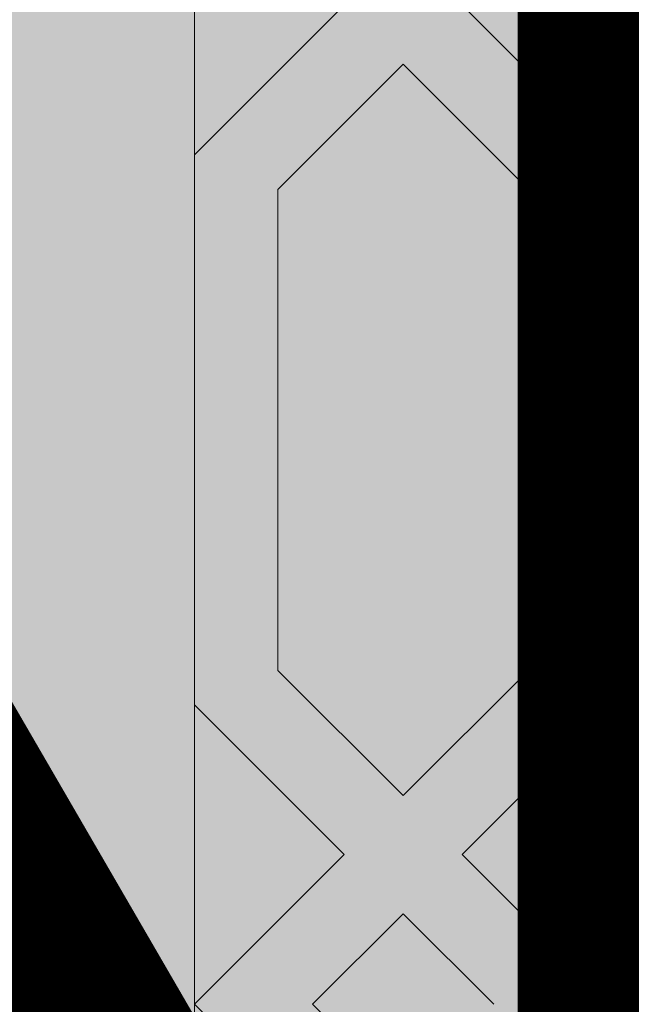
# Model space of a CAD drawing. Units: inches. Extents: x 844 to 2234, y 346 to 1084.
# Tile 83 of 93: x 2008.425 to 2010.294, y 701.365 to 704.373. Entities that reach past the tile are written whole.
import ezdxf

# ---------------------------------------------------------------- set-up
doc = ezdxf.new("R2010")
doc.units = ezdxf.units.IN
doc.header["$MEASUREMENT"] = 0
for name, color, linetype, lineweight in [('A-ANNO-DIMS', 2, 'Continuous', 18), ('furniture', 8, 'Continuous', 18), ('RA-AP-01$0$INT', 35, 'Continuous', 5)]:
    doc.layers.add(name, color=color, linetype=linetype, lineweight=lineweight)
doc.layers.add('RA-AP-01$0$FURN', color=3, linetype='Continuous')
doc.styles.get("Standard").update_dxf_attribs({"font": 'arial.ttf'})
doc.dimstyles.get("Standard").update_dxf_attribs({"dimtxt": 6, "dimasz": 3, "dimexe": 0.18, "dimexo": 0.0625, "dimgap": 0.09, "dimtad": 0, "dimtih": 1, "dimtoh": 1, "dimdec": 1, "dimzin": 0, "dimdsep": 46, "dimlunit": 3, "dimtxsty": 'Standard', "dimblk": 'ARCHTICK', "dimcen": 0.09, "dimadec": 0, "dimazin": 0, "dimtfac": 1, "dimtdec": 1, "dimtofl": 0, "dimtmove": 0, "dimatfit": 3, "dimfxl": 1, "dimtolj": 1, "dimtzin": 0, "dimarcsym": 0})

# ---------------------------------------------------------------- blocks, each defined once
blk = doc.blocks.new('A$C18D01794')
at = {"layer": 'RA-AP-01$0$INT'}
h = blk.add_hatch(color=256, dxfattribs=at)
h.paths.add_polyline_path([(4.35521, -6.15671), (4.35521, -8.05671), (5.45521, -8.05671), (5.45521, -6.15671)])
h.paths.add_polyline_path([(4.40521, -8.00671), (4.40521, -6.20671), (5.40521, -6.20671), (5.40521, -8.00671)], flags=16)
h = blk.add_hatch(color=256, dxfattribs=at)
h.paths.add_polyline_path([(4.46935, -7.07085), (4.50521, -7.035), (4.50521, -7.10671)])
h.paths.add_polyline_path([(4.45521, -7.085), (4.47692, -7.10671), (4.43349, -7.10671)])
h.paths.add_polyline_path([(4.40521, -7.035), (4.44106, -7.07085), (4.40521, -7.10671)])
h.paths.add_polyline_path([(4.42521, -6.91146), (4.45521, -6.88146), (4.48521, -6.91146), (4.48521, -7.02671), (4.45521, -7.05671), (4.42521, -7.02671)])
h.paths.add_polyline_path([(4.50521, -6.83146), (4.50521, -6.90318), (4.46935, -6.86732)])
h.paths.add_polyline_path([(4.42521, -6.70793), (4.45521, -6.67793), (4.48521, -6.70793), (4.48521, -6.82318), (4.45521, -6.85318), (4.42521, -6.82318)])
h.paths.add_polyline_path([(4.42521, -6.50439), (4.45521, -6.47439), (4.48521, -6.50439), (4.48521, -6.61964), (4.45521, -6.64964), (4.42521, -6.61964)])
h.paths.add_polyline_path([(4.46935, -6.66378), (4.50521, -6.62793), (4.50521, -6.69964)])
h.paths.add_polyline_path([(4.40521, -6.62793), (4.44106, -6.66378), (4.40521, -6.69964)])
h.paths.add_polyline_path([(4.40521, -6.42439), (4.44106, -6.46025), (4.40521, -6.49611)])
h.paths.add_polyline_path([(4.46935, -6.46025), (4.50521, -6.42439), (4.50521, -6.49611)])
h.paths.add_polyline_path([(4.42521, -6.30085), (4.45521, -6.27085), (4.48521, -6.30085), (4.48521, -6.41611), (4.45521, -6.44611), (4.42521, -6.41611)])
h.paths.add_polyline_path([(4.42521, -6.22671), (4.47106, -6.22671), (4.42521, -6.27257)])
h.paths.add_polyline_path([(4.49935, -6.22671), (4.63606, -6.22671), (4.66606, -6.25671), (4.63606, -6.28671), (4.49935, -6.28671), (4.46935, -6.25671)])
h.paths.add_polyline_path([(4.68021, -6.27085), (4.71606, -6.30671), (4.64435, -6.30671)])
h.paths.add_polyline_path([(4.64435, -6.20671), (4.71606, -6.20671), (4.68021, -6.24257)])
h.paths.add_polyline_path([(4.72435, -6.22671), (4.86106, -6.22671), (4.89106, -6.25671), (4.86106, -6.28671), (4.72435, -6.28671), (4.69435, -6.25671)])
h.paths.add_polyline_path([(4.90521, -6.27085), (4.94106, -6.30671), (4.86935, -6.30671)])
h.paths.add_polyline_path([(4.86935, -6.20671), (4.94106, -6.20671), (4.90521, -6.24257)])
h.paths.add_polyline_path([(4.94935, -6.22671), (5.08606, -6.22671), (5.11606, -6.25671), (5.08606, -6.28671), (4.94935, -6.28671), (4.91935, -6.25671)])
h.paths.add_polyline_path([(5.13021, -6.27085), (5.16606, -6.30671), (5.09435, -6.30671)])
h.paths.add_polyline_path([(5.09435, -6.20671), (5.16606, -6.20671), (5.13021, -6.24257)])
h.paths.add_polyline_path([(5.17435, -6.22671), (5.31106, -6.22671), (5.34106, -6.25671), (5.31106, -6.28671), (5.17435, -6.28671), (5.14435, -6.25671)])
h.paths.add_polyline_path([(5.32521, -6.30085), (5.35521, -6.27085), (5.38521, -6.30085), (5.38521, -6.41611), (5.35521, -6.44611), (5.32521, -6.41611)])
h.paths.add_polyline_path([(5.33935, -6.22671), (5.38521, -6.22671), (5.38521, -6.27257)])
h.paths.add_polyline_path([(5.32521, -6.50439), (5.35521, -6.47439), (5.38521, -6.50439), (5.38521, -6.61964), (5.35521, -6.64964), (5.32521, -6.61964)])
h.paths.add_polyline_path([(5.30521, -6.42439), (5.34106, -6.46025), (5.30521, -6.49611)])
h.paths.add_polyline_path([(5.36935, -6.46025), (5.40521, -6.42439), (5.40521, -6.49611)])
h.paths.add_polyline_path([(5.40521, -6.62793), (5.40521, -6.69964), (5.36935, -6.66378)])
h.paths.add_polyline_path([(5.30521, -6.62793), (5.34106, -6.66378), (5.30521, -6.69964)])
h.paths.add_polyline_path([(5.32521, -6.70793), (5.35521, -6.67793), (5.38521, -6.70793), (5.38521, -6.82318), (5.35521, -6.85318), (5.32521, -6.82318)])
h.paths.add_polyline_path([(5.30521, -6.83146), (5.34106, -6.86732), (5.30521, -6.90318)])
h.paths.add_polyline_path([(5.32521, -6.91146), (5.35521, -6.88146), (5.38521, -6.91146), (5.38521, -7.02671), (5.35521, -7.05671), (5.32521, -7.02671)])
h.paths.add_polyline_path([(5.40458, -6.83209, 0.001218), (5.40521, -6.83231), (5.40521, -6.90318), (5.36935, -6.86732)])
h.paths.add_polyline_path([(5.36935, -7.07085), (5.40521, -7.035), (5.40521, -7.10671)])
h.paths.add_polyline_path([(5.35521, -7.085), (5.37692, -7.10671), (5.33349, -7.10671)])
h.paths.add_polyline_path([(5.30521, -7.035), (5.34106, -7.07085), (5.30521, -7.10671)])
h = blk.add_hatch(color=256, dxfattribs=at)
h.paths.add_polyline_path([(4.50521, -6.62793), (4.46935, -6.66378), (4.50521, -6.69964), (4.50521, -6.83146), (4.46935, -6.86732), (4.50521, -6.90318), (4.50521, -7.035), (4.46935, -7.07085), (4.50521, -7.10671), (4.47692, -7.10671), (4.45521, -7.085), (4.43349, -7.10671), (4.40521, -7.10671), (4.44106, -7.07085), (4.40521, -7.035), (4.40521, -6.90318), (4.44106, -6.86732), (4.40521, -6.83146), (4.40521, -6.69964), (4.44106, -6.66378), (4.40521, -6.62793), (4.40521, -6.49611), (4.44106, -6.46025), (4.40521, -6.42439), (4.40521, -6.20671), (4.64435, -6.20671), (4.68021, -6.24257), (4.71606, -6.20671), (4.86935, -6.20671), (4.90521, -6.24257), (4.94106, -6.20671), (5.09435, -6.20671), (5.13021, -6.24257), (5.16606, -6.20671), (5.40521, -6.20671), (5.40521, -6.42439), (5.36935, -6.46025), (5.40521, -6.49611), (5.40521, -6.62793), (5.36935, -6.66378), (5.40521, -6.69964), (5.40521, -6.83146), (5.36935, -6.86732), (5.40521, -6.90318), (5.40521, -7.035), (5.36935, -7.07085), (5.40521, -7.10671), (5.37692, -7.10671), (5.35521, -7.085), (5.33349, -7.10671), (5.30521, -7.10671), (5.34106, -7.07085), (5.30521, -7.035), (5.30521, -6.90318), (5.34106, -6.86732), (5.30521, -6.83146), (5.30521, -6.69964), (5.34106, -6.66378), (5.30521, -6.62793), (5.30521, -6.49611), (5.34106, -6.46025), (5.30521, -6.42439), (5.30521, -6.30671), (5.16606, -6.30671), (5.13021, -6.27085), (5.09435, -6.30671), (4.94106, -6.30671), (4.90521, -6.27085), (4.86935, -6.30671), (4.71606, -6.30671), (4.68021, -6.27085), (4.64435, -6.30671), (4.50521, -6.30671), (4.50521, -6.42439), (4.46935, -6.46025), (4.50521, -6.49611)])
h.paths.add_polyline_path([(4.48521, -6.50439), (4.45521, -6.47439), (4.42521, -6.50439), (4.42521, -6.61964), (4.45521, -6.64964), (4.48521, -6.61964)], flags=16)
h.paths.add_polyline_path([(4.45521, -6.44611), (4.48521, -6.41611), (4.48521, -6.30085), (4.45521, -6.27085), (4.42521, -6.30085), (4.42521, -6.41611)], flags=16)
h.paths.add_polyline_path([(4.45521, -6.67793), (4.42521, -6.70793), (4.42521, -6.82318), (4.45521, -6.85318), (4.48521, -6.82318), (4.48521, -6.70793)], flags=16)
h.paths.add_polyline_path([(4.49935, -6.28671), (4.63606, -6.28671), (4.66606, -6.25671), (4.63606, -6.22671), (4.49935, -6.22671), (4.46935, -6.25671)], flags=16)
h.paths.add_polyline_path([(4.42521, -6.27257), (4.47106, -6.22671), (4.42521, -6.22671)], flags=16)
h.paths.add_polyline_path([(4.45521, -6.88146), (4.42521, -6.91146), (4.42521, -7.02671), (4.45521, -7.05671), (4.48521, -7.02671), (4.48521, -6.91146)], flags=16)
h.paths.add_polyline_path([(4.72435, -6.28671), (4.86106, -6.28671), (4.89106, -6.25671), (4.86106, -6.22671), (4.72435, -6.22671), (4.69435, -6.25671)], flags=16)
h.paths.add_polyline_path([(4.91935, -6.25671), (4.94935, -6.28671), (5.08606, -6.28671), (5.11606, -6.25671), (5.08606, -6.22671), (4.94935, -6.22671)], flags=16)
h.paths.add_polyline_path([(5.14435, -6.25671), (5.17435, -6.28671), (5.31106, -6.28671), (5.34106, -6.25671), (5.31106, -6.22671), (5.17435, -6.22671)], flags=16)
h.paths.add_polyline_path([(5.32521, -6.61964), (5.35521, -6.64964), (5.38521, -6.61964), (5.38521, -6.50439), (5.35521, -6.47439), (5.32521, -6.50439)], flags=16)
h.paths.add_polyline_path([(5.32521, -6.41611), (5.35521, -6.44611), (5.38521, -6.41611), (5.38521, -6.30085), (5.35521, -6.27085), (5.32521, -6.30085)], flags=16)
h.paths.add_polyline_path([(5.32521, -6.70793), (5.32521, -6.82318), (5.35521, -6.85318), (5.38521, -6.82318), (5.38521, -6.70793), (5.35521, -6.67793)], flags=16)
h.paths.add_polyline_path([(5.32521, -6.91146), (5.32521, -7.02671), (5.35521, -7.05671), (5.38521, -7.02671), (5.38521, -6.91146), (5.35521, -6.88146)], flags=16)
h.paths.add_polyline_path([(5.33935, -6.22671), (5.38521, -6.27257), (5.38521, -6.22671)], flags=16)
for points in [[(4.50521, -6.30671), (5.30521, -6.30671), (5.30521, -7.10671), (5.25521, -7.10671), (5.25521, -6.35671), (4.55521, -6.35671), (4.55521, -7.10671), (4.50521, -7.10671)], [(4.50521, -7.90671), (5.30521, -7.90671), (5.30521, -7.10671), (5.25521, -7.10671), (5.25521, -7.85671), (4.55521, -7.85671), (4.55521, -7.10671), (4.50521, -7.10671)], [(4.40521, -7.38196), (4.44106, -7.34611), (4.40521, -7.31025)]]:
    blk.add_hatch(color=256, dxfattribs=at).paths.add_polyline_path(points)
h = blk.add_hatch(color=256, dxfattribs=at)
h.paths.add_polyline_path([(4.50521, -7.5855), (4.46935, -7.54964), (4.50521, -7.51378), (4.50521, -7.38196), (4.46935, -7.34611), (4.50521, -7.31025), (4.50521, -7.17843), (4.46935, -7.14257), (4.50521, -7.10671), (4.47692, -7.10671), (4.45521, -7.12843), (4.43349, -7.10671), (4.40521, -7.10671), (4.44106, -7.14257), (4.40521, -7.17843), (4.40521, -7.31025), (4.44106, -7.34611), (4.40521, -7.38196), (4.40521, -7.51378), (4.44106, -7.54964), (4.40521, -7.5855), (4.40521, -7.71732), (4.44106, -7.75318), (4.40521, -7.78903), (4.40521, -8.00671), (4.64435, -8.00671), (4.68021, -7.97085), (4.71606, -8.00671), (4.86935, -8.00671), (4.90521, -7.97085), (4.94106, -8.00671), (5.09435, -8.00671), (5.13021, -7.97085), (5.16606, -8.00671), (5.40521, -8.00671), (5.40521, -7.78903), (5.36935, -7.75318), (5.40521, -7.71732), (5.40521, -7.5855), (5.36935, -7.54964), (5.40521, -7.51378), (5.40521, -7.38196), (5.36935, -7.34611), (5.40521, -7.31025), (5.40521, -7.17843), (5.36935, -7.14257), (5.40521, -7.10671), (5.37692, -7.10671), (5.35521, -7.12843), (5.33349, -7.10671), (5.30521, -7.10671), (5.34106, -7.14257), (5.30521, -7.17843), (5.30521, -7.31025), (5.34106, -7.34611), (5.30521, -7.38196), (5.30521, -7.51378), (5.34106, -7.54964), (5.30521, -7.5855), (5.30521, -7.71732), (5.34106, -7.75318), (5.30521, -7.78903), (5.30521, -7.90671), (5.16606, -7.90671), (5.13021, -7.94257), (5.09435, -7.90671), (4.94106, -7.90671), (4.90521, -7.94257), (4.86935, -7.90671), (4.71606, -7.90671), (4.68021, -7.94257), (4.64435, -7.90671), (4.50521, -7.90671), (4.50521, -7.78903), (4.46935, -7.75318), (4.50521, -7.71732)])
h.paths.add_polyline_path([(4.48521, -7.70903), (4.45521, -7.73903), (4.42521, -7.70903), (4.42521, -7.59378), (4.45521, -7.56378), (4.48521, -7.59378)], flags=16)
h.paths.add_polyline_path([(4.45521, -7.76732), (4.48521, -7.79732), (4.48521, -7.91257), (4.45521, -7.94257), (4.42521, -7.91257), (4.42521, -7.79732)], flags=16)
h.paths.add_polyline_path([(4.45521, -7.5355), (4.42521, -7.5055), (4.42521, -7.39025), (4.45521, -7.36025), (4.48521, -7.39025), (4.48521, -7.5055)], flags=16)
h.paths.add_polyline_path([(4.49935, -7.92671), (4.63606, -7.92671), (4.66606, -7.95671), (4.63606, -7.98671), (4.49935, -7.98671), (4.46935, -7.95671)], flags=16)
h.paths.add_polyline_path([(4.42521, -7.94085), (4.47106, -7.98671), (4.42521, -7.98671)], flags=16)
h.paths.add_polyline_path([(4.45521, -7.33196), (4.42521, -7.30196), (4.42521, -7.18671), (4.45521, -7.15671), (4.48521, -7.18671), (4.48521, -7.30196)], flags=16)
h.paths.add_polyline_path([(4.72435, -7.92671), (4.86106, -7.92671), (4.89106, -7.95671), (4.86106, -7.98671), (4.72435, -7.98671), (4.69435, -7.95671)], flags=16)
h.paths.add_polyline_path([(4.91935, -7.95671), (4.94935, -7.92671), (5.08606, -7.92671), (5.11606, -7.95671), (5.08606, -7.98671), (4.94935, -7.98671)], flags=16)
h.paths.add_polyline_path([(5.14435, -7.95671), (5.17435, -7.92671), (5.31106, -7.92671), (5.34106, -7.95671), (5.31106, -7.98671), (5.17435, -7.98671)], flags=16)
h.paths.add_polyline_path([(5.32521, -7.59378), (5.35521, -7.56378), (5.38521, -7.59378), (5.38521, -7.70903), (5.35521, -7.73903), (5.32521, -7.70903)], flags=16)
h.paths.add_polyline_path([(5.32521, -7.79732), (5.35521, -7.76732), (5.38521, -7.79732), (5.38521, -7.91257), (5.35521, -7.94257), (5.32521, -7.91257)], flags=16)
h.paths.add_polyline_path([(5.32521, -7.5055), (5.32521, -7.39025), (5.35521, -7.36025), (5.38521, -7.39025), (5.38521, -7.5055), (5.35521, -7.5355)], flags=16)
h.paths.add_polyline_path([(5.32521, -7.30196), (5.32521, -7.18671), (5.35521, -7.15671), (5.38521, -7.18671), (5.38521, -7.30196), (5.35521, -7.33196)], flags=16)
h.paths.add_polyline_path([(5.33935, -7.98671), (5.38521, -7.94085), (5.38521, -7.98671)], flags=16)
h = blk.add_hatch(color=256, dxfattribs=at)
h.paths.add_polyline_path([(4.46935, -7.14257), (4.50521, -7.17843), (4.50521, -7.10671)])
h.paths.add_polyline_path([(4.45521, -7.12843), (4.47692, -7.10671), (4.43349, -7.10671)])
h.paths.add_polyline_path([(4.40521, -7.17843), (4.44106, -7.14257), (4.40521, -7.10671)])
h.paths.add_polyline_path([(4.42521, -7.30196), (4.45521, -7.33196), (4.48521, -7.30196), (4.48521, -7.18671), (4.45521, -7.15671), (4.42521, -7.18671)])
h.paths.add_polyline_path([(4.50521, -7.38196), (4.50521, -7.31025), (4.46935, -7.34611)])
h.paths.add_polyline_path([(4.42521, -7.5055), (4.45521, -7.5355), (4.48521, -7.5055), (4.48521, -7.39025), (4.45521, -7.36025), (4.42521, -7.39025)])
h.paths.add_polyline_path([(4.42521, -7.70903), (4.45521, -7.73903), (4.48521, -7.70903), (4.48521, -7.59378), (4.45521, -7.56378), (4.42521, -7.59378)])
h.paths.add_polyline_path([(4.46935, -7.54964), (4.50521, -7.5855), (4.50521, -7.51378)])
h.paths.add_polyline_path([(4.40521, -7.5855), (4.44106, -7.54964), (4.40521, -7.51378)])
h.paths.add_polyline_path([(4.40521, -7.78903), (4.44106, -7.75318), (4.40521, -7.71732)])
h.paths.add_polyline_path([(4.46935, -7.75318), (4.50521, -7.78903), (4.50521, -7.71732)])
h.paths.add_polyline_path([(4.42521, -7.91257), (4.45521, -7.94257), (4.48521, -7.91257), (4.48521, -7.79732), (4.45521, -7.76732), (4.42521, -7.79732)])
h.paths.add_polyline_path([(4.42521, -7.98671), (4.47106, -7.98671), (4.42521, -7.94085)])
h.paths.add_polyline_path([(4.49935, -7.98671), (4.63606, -7.98671), (4.66606, -7.95671), (4.63606, -7.92671), (4.49935, -7.92671), (4.46935, -7.95671)])
h.paths.add_polyline_path([(4.68021, -7.94257), (4.71606, -7.90671), (4.64435, -7.90671)])
h.paths.add_polyline_path([(4.64435, -8.00671), (4.71606, -8.00671), (4.68021, -7.97085)])
h.paths.add_polyline_path([(4.72435, -7.98671), (4.86106, -7.98671), (4.89106, -7.95671), (4.86106, -7.92671), (4.72435, -7.92671), (4.69435, -7.95671)])
h.paths.add_polyline_path([(4.90521, -7.94257), (4.94106, -7.90671), (4.86935, -7.90671)])
h.paths.add_polyline_path([(4.86935, -8.00671), (4.94106, -8.00671), (4.90521, -7.97085)])
h.paths.add_polyline_path([(4.94935, -7.98671), (5.08606, -7.98671), (5.11606, -7.95671), (5.08606, -7.92671), (4.94935, -7.92671), (4.91935, -7.95671)])
h.paths.add_polyline_path([(5.13021, -7.94257), (5.16606, -7.90671), (5.09435, -7.90671)])
h.paths.add_polyline_path([(5.09435, -8.00671), (5.16606, -8.00671), (5.13021, -7.97085)])
h.paths.add_polyline_path([(5.17435, -7.98671), (5.31106, -7.98671), (5.34106, -7.95671), (5.31106, -7.92671), (5.17435, -7.92671), (5.14435, -7.95671)])
h.paths.add_polyline_path([(5.32521, -7.91257), (5.35521, -7.94257), (5.38521, -7.91257), (5.38521, -7.79732), (5.35521, -7.76732), (5.32521, -7.79732)])
h.paths.add_polyline_path([(5.33935, -7.98671), (5.38521, -7.98671), (5.38521, -7.94085)])
h.paths.add_polyline_path([(5.32521, -7.70903), (5.35521, -7.73903), (5.38521, -7.70903), (5.38521, -7.59378), (5.35521, -7.56378), (5.32521, -7.59378)])
h.paths.add_polyline_path([(5.30521, -7.78903), (5.34106, -7.75318), (5.30521, -7.71732)])
h.paths.add_polyline_path([(5.36935, -7.75318), (5.40521, -7.78903), (5.40521, -7.71732)])
h.paths.add_polyline_path([(5.40521, -7.5855), (5.40521, -7.51378), (5.36935, -7.54964)])
h.paths.add_polyline_path([(5.30521, -7.5855), (5.34106, -7.54964), (5.30521, -7.51378)])
h.paths.add_polyline_path([(5.32521, -7.5055), (5.35521, -7.5355), (5.38521, -7.5055), (5.38521, -7.39025), (5.35521, -7.36025), (5.32521, -7.39025)])
h.paths.add_polyline_path([(5.30521, -7.38196), (5.34106, -7.34611), (5.30521, -7.31025)])
h.paths.add_polyline_path([(5.32521, -7.30196), (5.35521, -7.33196), (5.38521, -7.30196), (5.38521, -7.18671), (5.35521, -7.15671), (5.32521, -7.18671)])
h.paths.add_polyline_path([(5.40458, -7.38134, -0.001218), (5.40521, -7.38111), (5.40521, -7.31025), (5.36935, -7.34611)])
h.paths.add_polyline_path([(5.36935, -7.14257), (5.40521, -7.17843), (5.40521, -7.10671)])
h.paths.add_polyline_path([(5.35521, -7.12843), (5.37692, -7.10671), (5.33349, -7.10671)])
h.paths.add_polyline_path([(5.30521, -7.17843), (5.34106, -7.14257), (5.30521, -7.10671)])
for p, q in [((4.46935, -7.07085), (4.50521, -7.10671)), ((4.45521, -7.085), (4.47692, -7.10671)), ((4.44106, -7.14257), (4.40521, -7.10671)), ((4.45521, -7.12843), (4.43349, -7.10671)), ((4.45521, -7.12843), (4.47692, -7.10671)), ((4.46935, -7.14257), (4.50521, -7.10671)), ((4.40521, -7.17843), (4.44106, -7.14257)), ((4.50521, -7.17843), (4.46935, -7.14257)), ((4.42521, -7.18671), (4.45521, -7.15671)), ((4.48521, -7.18671), (4.45521, -7.15671)), ((4.42521, -7.30196), (4.42521, -7.18671)), ((4.48521, -7.30196), (4.48521, -7.18671)), ((4.42521, -7.30196), (4.45521, -7.33196)), ((4.48521, -7.30196), (4.45521, -7.33196)), ((4.40521, -7.31025), (4.44106, -7.34611)), ((4.50521, -7.31025), (4.46935, -7.34611))]:
    blk.add_line(p, q, dxfattribs=at)
for points in [[(5.30521, -7.10671), (5.30521, -6.30671), (4.50521, -6.30671), (4.50521, -7.10671)], [(5.40521, -8.00671), (4.40521, -8.00671), (4.40521, -7.10671)], [(5.30521, -7.10671), (5.30521, -7.90671), (4.50521, -7.90671), (4.50521, -7.10671)]]:
    blk.add_lwpolyline(points, dxfattribs=at)
blk = doc.blocks.new('A$C5D2F253E')
at = {"layer": 'RA-AP-01$0$FURN', "xscale": -0.7999999999883585, "yscale": 0.7999999999883585, "zscale": 0.8, "rotation": 90}
blk.add_blockref('A$C18D01794', (-5.68776, 4.75792), dxfattribs=at)
blk = doc.blocks.new('_ArchTick')
at = {"color": 0, "linetype": 'ByBlock', "const_width": 0.15}
blk.add_lwpolyline([(-0.5, -0.5), (0.5, 0.5)], dxfattribs=at)
blk = doc.blocks.new('*D121')
at = {"layer": 'A-ANNO-DIMS', "color": 0, "lineweight": -2, "transparency": 16777216}
for p, q in [((2030.272, 734.2626), (2040.2453, 734.2626)), ((2040.0653, 734.2626), (2040.0653, 704.6044)), ((2040.0653, 668.5574), (2040.0653, 698.2156)), ((2030.272, 668.5574), (2040.2453, 668.5574))]:
    blk.add_line(p, q, dxfattribs=at)
at = {"layer": 'Defpoints', "color": 0, "transparency": 16777216}
for p in [(2030.2095, 734.2626), (2040.0653, 734.2626), (2030.2095, 668.5574)]:
    blk.add_point(p, dxfattribs=at)
at = {"layer": 'A-ANNO-DIMS', "color": 0, "lineweight": -2, "transparency": 16777216, "xscale": 3, "yscale": 3, "zscale": 3}
for p, rotation in [((2040.0653, 734.2626), 90), ((2040.0653, 668.5574), 270)]:
    blk.add_blockref('_ArchTick', p, dxfattribs=dict(at, rotation=rotation))
at = {"layer": 'A-ANNO-DIMS', "color": 0, "transparency": 16777216, "insert": (2040.0653, 701.41), "char_height": 6, "attachment_point": 5}
blk.add_mtext('\\A1;LOUNGE SET 5\'-5 1/2" TYP.', dxfattribs=at)

msp = doc.modelspace()

# ---------------------------------------------------------------- block references
at = {"layer": 'furniture', "xscale": -15.94108302203742, "yscale": 15.94108302203742, "zscale": 15.94108302203742, "rotation": 270}
msp.add_blockref('A$C5D2F253E', (1990.5673, 701.4029), dxfattribs=at)

# ---------------------------------------------------------------- dimensions: what is measured, and where the dimension line sits
at = {"layer": 'A-ANNO-DIMS'}
dim = msp.add_linear_dim(base=(2040.0653, 734.2626), p1=(2030.2095, 668.5574), p2=(2030.2095, 734.2626), angle=90, text='LOUNGE SET <> TYP.', dimstyle='Standard', override={"dimdec": 1, "dimlfac": 1, "dimrnd": 0, "dimzin": 1, "dimdsep": 46, "dimlunit": 4, "dimfrac": 2}, dxfattribs=at)
dim.commit()
dim.dimension.update_dxf_attribs({"geometry": '*D121', "text_midpoint": (2040.0653, 701.41)})

doc.saveas('drawing.dxf')
